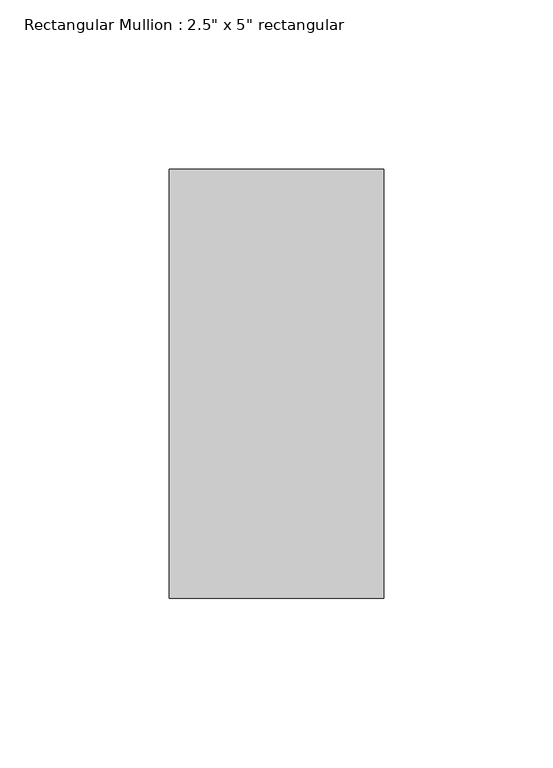
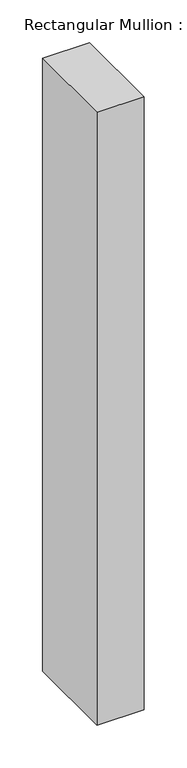
"""IFC4 building model written with IfcOpenShell, lengths in millimetres: member geometry."""

from ifc_helpers import new_model, si_unit, frame, origin, place, context, project, spatial, polyline, outline, extrude, source, transform, mapped, element, save


def member_ac493aea(model_context):
    return source(origin(), model_context, "Body", "SweptSolid", [
        extrude(outline(polyline([(0.0, 63.5), (0.0, -63.5), (-63.5, -63.5), (-63.5, 63.5), (0.0, 63.5)])), frame((0.0, 0.0, -873.5902035), z_axis=(0.0, 0.0, 1.0), x_axis=(1.0, 0.0, 0.0)), (0.0, 0.0, 1.0), 873.5902035),
    ])


if __name__ == "__main__":
    model = new_model("IFC4")
    model_context = context("Model", 3, world=origin())
    ifc_project = project(units=[si_unit("LENGTHUNIT", "METRE", prefix="MILLI")], contexts=[model_context])
    site = spatial("IfcSite", under=ifc_project)
    building = spatial("IfcBuilding", under=site)
    placement = place(None, origin())
    member_shape = member_ac493aea(model_context)
    element("IfcMember", 1, ObjectType="Rectangular Mullion : 2.5\" x 5\" rectangular", at=placement, inside=building, context=model_context, shape_type="MappedRepresentation", body=[
        mapped(member_shape, transform((0.0, 0.0, 0.0), x_axis=(1.0, 0.0, 0.0), y_axis=(0.0, 1.0, 0.0), z_axis=(0.0, 0.0, 1.0))),
    ])
    save(model, "model.ifc")

# Revit data of these elements
# Type "Rectangular Mullion : 2.5\" x 5\" rectangular"
#   built-in parameter 1007304 = 0.416667 (stored number, unit not read)
#   built-in parameter 1007301 = 0.104167 (stored number, unit not read)
#   built-in parameter 1007300 = 0.104167 (stored number, unit not read)
# Element 1 (IfcMember, "Rectangular Mullion : 2.5\" x 5\" rectangular")
#   Materials on its faces: "Aluminum"
# Materials
#   "Aluminum": class "Metal", colour RGB 247 247 247, transparency 0, Description = "Aluminum 6061", Cost = 0
